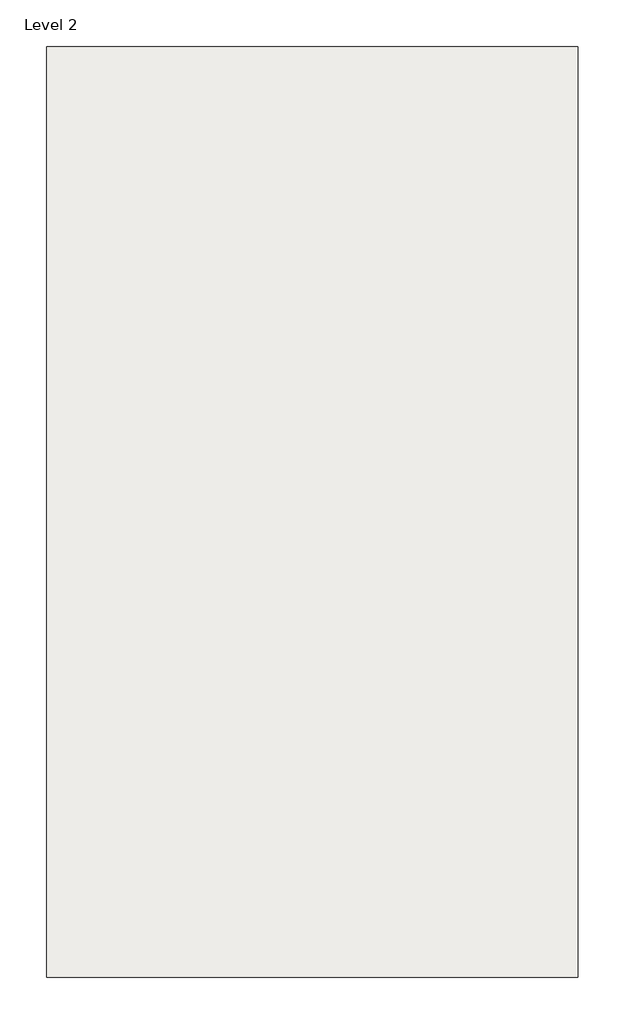
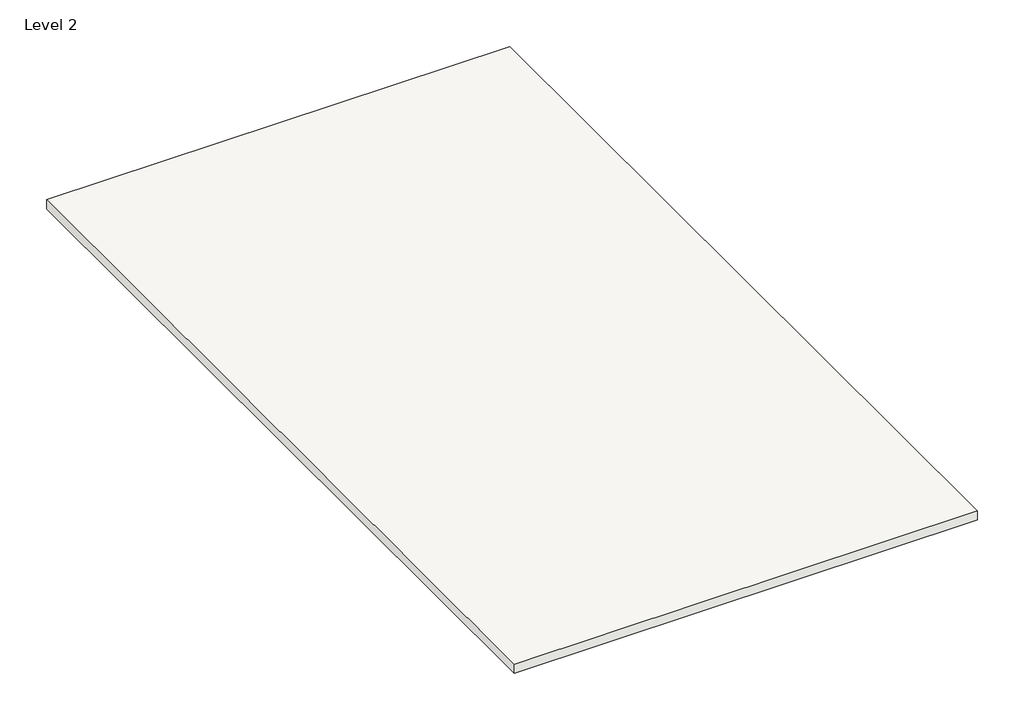
# One storey: 1 roof.
"""IFC4 building model written with IfcOpenShell, lengths in millimetres."""

from ifc_helpers import new_model, si_unit, frame, origin, place, context, project, spatial, polyline, outline, extrude, element, save

model = new_model("IFC4")

# Units and contexts
model_context = context("Model", 3, world=origin())
ifc_project = project(units=[si_unit("LENGTHUNIT", "METRE", prefix="MILLI")], contexts=[model_context])

# Site, building, storey
site = spatial("IfcSite", under=ifc_project)
building = spatial("IfcBuilding", under=site)
storey = spatial("IfcBuildingStorey", under=building, Name="Level 2", Elevation=3048.0)

# Roof
placement = place(None, origin())
element("IfcRoof", 1, ObjectType="Generic - 12\"", at=placement, inside=storey, context=model_context, shape_type="SweptSolid", body=[
    extrude(outline(polyline([(1016.0, 14452.6), (8331.2, 14452.6), (8331.2, 1651.0), (1016.0, 1651.0), (1016.0, 14452.6)])), frame((0.0, 0.0, 3048.0), z_axis=(0.0, 0.0, 1.0), x_axis=(1.0, 0.0, 0.0)), (0.0, 0.0, 1.0), 152.4),
])

save(model, "model.ifc")

# Revit data of these elements
# Type "Generic - 12\""
#   Assembly Code = "B1020"
#   Layers, outside or top first: 0' - 6" "Door - Panel" (function 1)
# Element 1 (IfcRoof, "Generic - 12\"")
#   built-in parameter 1001705 = 10.5 (stored number, unit not read)
#   built-in parameter 1001710 = 33615
#   Phase Created = New Construction
#   Materials on its faces: "Door - Panel"
# Materials
#   "Door - Panel": class "Wood", colour RGB 210 159 95, transparency 0, Cost = 0
